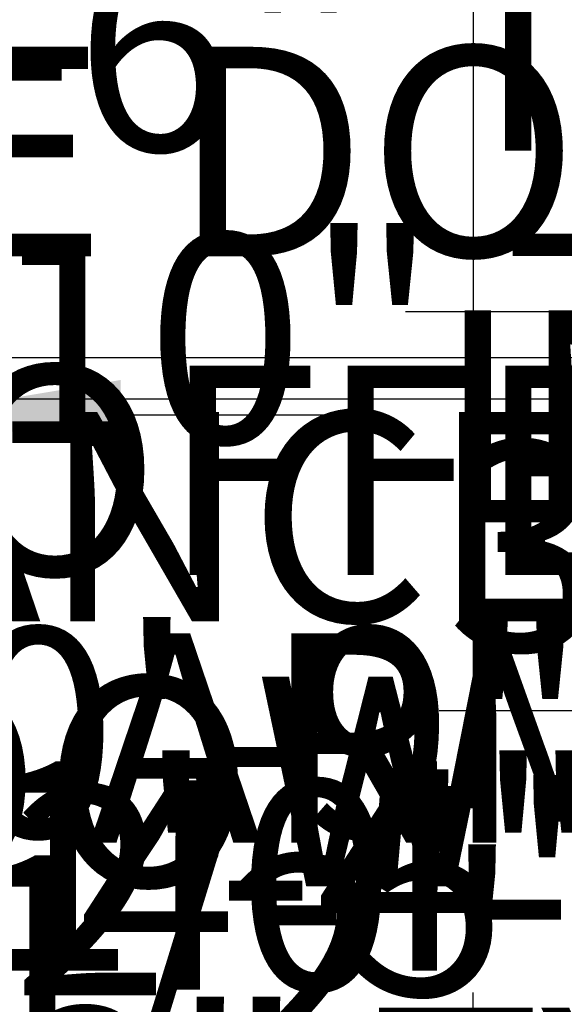
# Model space of a CAD drawing. Units: inches. Extents: x 7323 to 9737, y 2037 to 3322.
# Tile 9 of 19: x 8921 to 8999, y 2426 to 2568. Entities that reach past the tile are written whole.
import ezdxf

# ---------------------------------------------------------------- set-up
doc = ezdxf.new("R2010")
doc.units = ezdxf.units.IN
doc.header["$MEASUREMENT"] = 0
doc.layers.add('A-ANNO-DIMS', color=2, linetype='Continuous', lineweight=18)
doc.styles.get("Standard").update_dxf_attribs({"font": 'arial.ttf'})
doc.dimstyles.get("Standard").update_dxf_attribs({"dimtxt": 30.18, "dimasz": 30.18, "dimexe": 0.18, "dimexo": 0.0625, "dimgap": 0.09, "dimtad": 0, "dimtih": 1, "dimtoh": 1, "dimdec": 0, "dimzin": 0, "dimdsep": 46, "dimlunit": 3, "dimtxsty": 'Standard', "dimcen": 0.09, "dimadec": 0, "dimazin": 0, "dimtfac": 1, "dimtdec": 0, "dimtofl": 0, "dimtmove": 0, "dimatfit": 3, "dimfxl": 1, "dimtolj": 1, "dimtzin": 0, "dimarcsym": 0})

# ---------------------------------------------------------------- blocks, each defined once
blk = doc.blocks.new('*D11')
at = {"layer": 'A-ANNO-DIMS', "color": 0, "lineweight": -2, "transparency": 16777216}
for p, q in [((9007.88, 2687.3), (8985.8, 2687.3)), ((8985.98, 2657.12), (8985.98, 2458.79)), ((8985.98, 2229.48), (8985.98, 2427.8)), ((9007.88, 2199.3), (8985.8, 2199.3))]:
    blk.add_line(p, q, dxfattribs=at)
at = {"layer": 'A-ANNO-DIMS', "color": 0, "transparency": 16777216}
for points in [[(8980.95, 2657.12), (8991.01, 2657.12), (8985.98, 2687.3)], [(8980.95, 2229.48), (8991.01, 2229.48), (8985.98, 2199.3)]]:
    blk.add_solid(points, dxfattribs=at)
at = {"layer": 'Defpoints', "color": 0, "transparency": 16777216}
for p in [(9007.95, 2687.3), (8985.98, 2199.3), (9007.95, 2199.3)]:
    blk.add_point(p, dxfattribs=at)
at = {"layer": 'A-ANNO-DIMS', "color": 0, "transparency": 16777216, "insert": (8985.98, 2443.3), "char_height": 30.18, "attachment_point": 5}
blk.add_mtext('\\A1;40\'-8"', dxfattribs=at)
blk = doc.blocks.new('*D39')
at = {"layer": 'A-ANNO-DIMS', "color": 0, "lineweight": -2, "transparency": 16777216}
for p, q in [((8647.94, 2549.03), (8617.76, 2549.03)), ((8678.12, 2543.2), (8678.12, 2549.21)), ((8717.39, 2543.2), (8717.39, 2549.21)), ((8747.57, 2549.03), (8777.75, 2549.03))]:
    blk.add_line(p, q, dxfattribs=at)
at = {"layer": 'A-ANNO-DIMS', "color": 0, "transparency": 16777216}
for points in [[(8647.94, 2554.06), (8647.94, 2544), (8678.12, 2549.03)], [(8747.57, 2554.06), (8747.57, 2544), (8717.39, 2549.03)]]:
    blk.add_solid(points, dxfattribs=at)
at = {"layer": 'Defpoints', "color": 0, "transparency": 16777216}
for p in [(8717.39, 2549.03), (8678.12, 2543.14), (8717.39, 2543.14)]:
    blk.add_point(p, dxfattribs=at)
at = {"layer": 'A-ANNO-DIMS', "color": 0, "transparency": 16777216, "insert": (9057.19, 2549.03), "char_height": 30.18, "attachment_point": 5}
blk.add_mtext('\\A1;SINGLE DOOR 3\'-3 1/2" TYP.', dxfattribs=at)
blk = doc.blocks.new('*D41')
at = {"layer": 'A-ANNO-DIMS', "color": 0, "lineweight": -2, "transparency": 16777216}
for p, q in [((8661.59, 2428.04), (8661.59, 2458.22)), ((8661.59, 2458.22), (8691.77, 2458.22)), ((8657.46, 2397.86), (8661.77, 2397.86)), ((8657.46, 2369.86), (8661.77, 2369.86)), ((8661.59, 2339.68), (8661.59, 2309.5))]:
    blk.add_line(p, q, dxfattribs=at)
at = {"layer": 'A-ANNO-DIMS', "color": 0, "transparency": 16777216}
for points in [[(8656.56, 2428.04), (8666.62, 2428.04), (8661.59, 2397.86)], [(8656.56, 2339.68), (8666.62, 2339.68), (8661.59, 2369.86)]]:
    blk.add_solid(points, dxfattribs=at)
at = {"layer": 'Defpoints', "color": 0, "transparency": 16777216}
for p in [(8657.39, 2397.86), (8661.59, 2397.86), (8657.39, 2369.86)]:
    blk.add_point(p, dxfattribs=at)
at = {"layer": 'A-ANNO-DIMS', "color": 0, "transparency": 16777216, "insert": (8945.06, 2458.22), "char_height": 30.18, "attachment_point": 5}
blk.add_mtext('\\A1;VENT WINDOW 2\'-4" TYP.', dxfattribs=at)
blk = doc.blocks.new('*D43')
at = {"layer": 'A-ANNO-DIMS', "color": 0, "lineweight": -2, "transparency": 16777216}
for p, q in [((9108.94, 2438.75), (9108.94, 2468.93)), ((9104.01, 2408.57), (9109.12, 2408.57)), ((9104.01, 2375.3), (9109.12, 2375.3)), ((9108.94, 2345.12), (9108.94, 2314.94))]:
    blk.add_line(p, q, dxfattribs=at)
at = {"layer": 'A-ANNO-DIMS', "color": 0, "transparency": 16777216}
for points in [[(9103.91, 2438.75), (9113.97, 2438.75), (9108.94, 2408.57)], [(9103.91, 2345.12), (9113.97, 2345.12), (9108.94, 2375.3)]]:
    blk.add_solid(points, dxfattribs=at)
at = {"layer": 'Defpoints', "color": 0, "transparency": 16777216}
for p in [(9103.95, 2408.57), (9108.94, 2408.57), (9103.95, 2375.3)]:
    blk.add_point(p, dxfattribs=at)
at = {"layer": 'A-ANNO-DIMS', "color": 0, "transparency": 16777216, "insert": (9108.94, 2391.93), "char_height": 30.18, "attachment_point": 5}
blk.add_mtext('\\A1;BATH DOOR 2\'-9 1/2" TYP.', dxfattribs=at)
blk = doc.blocks.new('*D47')
at = {"layer": 'A-ANNO-DIMS', "color": 0, "lineweight": -2, "transparency": 16777216}
for p, q in [((8809.55, 2464.49), (8779.37, 2464.49)), ((8839.73, 2461.79), (8839.73, 2464.67)), ((8858.14, 2461.79), (8858.14, 2464.67)), ((8888.32, 2464.49), (8918.5, 2464.49))]:
    blk.add_line(p, q, dxfattribs=at)
at = {"layer": 'A-ANNO-DIMS', "color": 0, "transparency": 16777216}
for points in [[(8809.55, 2469.52), (8809.55, 2459.46), (8839.73, 2464.49)], [(8888.32, 2469.52), (8888.32, 2459.46), (8858.14, 2464.49)]]:
    blk.add_solid(points, dxfattribs=at)
at = {"layer": 'Defpoints', "color": 0, "transparency": 16777216}
for p in [(8858.14, 2464.49), (8839.73, 2461.73), (8858.14, 2461.73)]:
    blk.add_point(p, dxfattribs=at)
at = {"layer": 'A-ANNO-DIMS', "color": 0, "transparency": 16777216, "insert": (9164.9, 2464.49), "char_height": 30.18, "attachment_point": 5}
blk.add_mtext('\\A1;ARMCHAIR 1\'-6 1/2" TYP.', dxfattribs=at)
blk = doc.blocks.new('*D48')
at = {"layer": 'A-ANNO-DIMS', "color": 0, "lineweight": -2, "transparency": 16777216}
for p, q in [((8836.96, 2491.91), (8836.96, 2522.09)), ((8836.96, 2522.09), (8867.14, 2522.09)), ((8839.66, 2461.73), (8836.78, 2461.73)), ((8839.66, 2451.75), (8836.78, 2451.75)), ((8836.96, 2421.57), (8836.96, 2391.39))]:
    blk.add_line(p, q, dxfattribs=at)
at = {"layer": 'A-ANNO-DIMS', "color": 0, "transparency": 16777216}
for points in [[(8831.93, 2491.91), (8841.99, 2491.91), (8836.96, 2461.73)], [(8831.93, 2421.57), (8841.99, 2421.57), (8836.96, 2451.75)]]:
    blk.add_solid(points, dxfattribs=at)
at = {"layer": 'Defpoints', "color": 0, "transparency": 16777216}
for p in [(8836.96, 2461.73), (8839.73, 2461.73), (8839.73, 2451.75)]:
    blk.add_point(p, dxfattribs=at)
at = {"layer": 'A-ANNO-DIMS', "color": 0, "transparency": 16777216, "insert": (8970.94, 2522.09), "char_height": 30.18, "attachment_point": 5}
blk.add_mtext('\\A1;0\'-10" TYP.', dxfattribs=at)
blk = doc.blocks.new('*D53')
at = {"layer": 'A-ANNO-DIMS', "color": 0, "lineweight": -2, "transparency": 16777216}
for p, q in [((8826.85, 2511.06), (8796.67, 2511.06)), ((8857.03, 2503.93), (8857.03, 2511.24)), ((8905.03, 2503.93), (8905.03, 2511.24)), ((8935.21, 2511.06), (8965.39, 2511.06))]:
    blk.add_line(p, q, dxfattribs=at)
at = {"layer": 'A-ANNO-DIMS', "color": 0, "transparency": 16777216}
for points in [[(8826.85, 2516.09), (8826.85, 2506.03), (8857.03, 2511.06)], [(8935.21, 2516.09), (8935.21, 2506.03), (8905.03, 2511.06)]]:
    blk.add_solid(points, dxfattribs=at)
at = {"layer": 'Defpoints', "color": 0, "transparency": 16777216}
for p in [(8905.03, 2511.06), (8857.03, 2503.86), (8905.03, 2503.86)]:
    blk.add_point(p, dxfattribs=at)
at = {"layer": 'A-ANNO-DIMS', "color": 0, "transparency": 16777216, "insert": (9261.3, 2511.06), "char_height": 30.18, "attachment_point": 5}
blk.add_mtext('\\A1;INTERIOR WINDOW 4\'-0" TYP.', dxfattribs=at)
blk = doc.blocks.new('*D54')
at = {"layer": 'A-ANNO-DIMS', "color": 0, "lineweight": -2, "transparency": 16777216}
for p, q in [((8849.83, 2534.04), (8849.83, 2564.22)), ((8849.83, 2564.22), (8880.01, 2564.22)), ((8856.96, 2503.86), (8849.65, 2503.86)), ((8856.96, 2497.86), (8849.65, 2497.86)), ((8849.83, 2467.68), (8849.83, 2437.5))]:
    blk.add_line(p, q, dxfattribs=at)
at = {"layer": 'A-ANNO-DIMS', "color": 0, "transparency": 16777216}
for points in [[(8844.8, 2534.04), (8854.86, 2534.04), (8849.83, 2503.86)], [(8844.8, 2467.68), (8854.86, 2467.68), (8849.83, 2497.86)]]:
    blk.add_solid(points, dxfattribs=at)
at = {"layer": 'Defpoints', "color": 0, "transparency": 16777216}
for p in [(8849.83, 2503.86), (8857.03, 2503.86), (8857.03, 2497.86)]:
    blk.add_point(p, dxfattribs=at)
at = {"layer": 'A-ANNO-DIMS', "color": 0, "transparency": 16777216, "insert": (8972.08, 2564.22), "char_height": 30.18, "attachment_point": 5}
blk.add_mtext('\\A1;0\'-6" TYP.', dxfattribs=at)
blk = doc.blocks.new('*D60')
at = {"layer": 'A-ANNO-DIMS', "color": 0, "lineweight": -2, "transparency": 16777216}
for p, q in [((9109.84, 2540.48), (9109.84, 2570.66)), ((9104.01, 2510.3), (9110.02, 2510.3)), ((9104.01, 2474.02), (9110.02, 2474.02)), ((9109.84, 2443.84), (9109.84, 2413.66))]:
    blk.add_line(p, q, dxfattribs=at)
at = {"layer": 'A-ANNO-DIMS', "color": 0, "transparency": 16777216}
for points in [[(9104.81, 2540.48), (9114.87, 2540.48), (9109.84, 2510.3)], [(9104.81, 2443.84), (9114.87, 2443.84), (9109.84, 2474.02)]]:
    blk.add_solid(points, dxfattribs=at)
at = {"layer": 'Defpoints', "color": 0, "transparency": 16777216}
for p in [(9103.95, 2510.3), (9109.84, 2510.3), (9103.95, 2474.02)]:
    blk.add_point(p, dxfattribs=at)
at = {"layer": 'A-ANNO-DIMS', "color": 0, "transparency": 16777216, "insert": (9109.84, 2492.16), "char_height": 30.18, "attachment_point": 5}
blk.add_mtext('\\A1;3\'-0 1/2" TYP.', dxfattribs=at)
blk = doc.blocks.new('*D63')
at = {"layer": 'A-ANNO-DIMS', "color": 0, "lineweight": -2, "transparency": 16777216}
for p, q in [((8744.72, 2466.22), (8744.72, 2496.4)), ((8744.72, 2496.4), (8774.9, 2496.4)), ((8741.46, 2436.04), (8744.9, 2436.04)), ((8741.46, 2413.86), (8744.9, 2413.86)), ((8744.72, 2383.68), (8744.72, 2353.5))]:
    blk.add_line(p, q, dxfattribs=at)
at = {"layer": 'A-ANNO-DIMS', "color": 0, "transparency": 16777216}
for points in [[(8739.69, 2466.22), (8749.75, 2466.22), (8744.72, 2436.04)], [(8739.69, 2383.68), (8749.75, 2383.68), (8744.72, 2413.86)]]:
    blk.add_solid(points, dxfattribs=at)
at = {"layer": 'Defpoints', "color": 0, "transparency": 16777216}
for p in [(8741.39, 2436.04), (8744.72, 2436.04), (8741.39, 2413.86)]:
    blk.add_point(p, dxfattribs=at)
at = {"layer": 'A-ANNO-DIMS', "color": 0, "transparency": 16777216, "insert": (9003.76, 2496.4), "char_height": 30.18, "attachment_point": 5}
blk.add_mtext('\\A1;APPLIANCE 1\'-10" TYP.', dxfattribs=at)
blk = doc.blocks.new('*D64')
at = {"layer": 'A-ANNO-DIMS', "color": 0, "lineweight": -2, "transparency": 16777216}
for p, q in [((8719.69, 2413.8), (8719.69, 2410.36)), ((8741.39, 2413.8), (8741.39, 2410.36)), ((8689.51, 2410.54), (8659.33, 2410.54)), ((8771.57, 2410.54), (8801.75, 2410.54))]:
    blk.add_line(p, q, dxfattribs=at)
at = {"layer": 'A-ANNO-DIMS', "color": 0, "transparency": 16777216}
for points in [[(8689.51, 2415.57), (8689.51, 2405.51), (8719.69, 2410.54)], [(8771.57, 2415.57), (8771.57, 2405.51), (8741.39, 2410.54)]]:
    blk.add_solid(points, dxfattribs=at)
at = {"layer": 'Defpoints', "color": 0, "transparency": 16777216}
for p in [(8719.69, 2413.86), (8741.39, 2413.86), (8741.39, 2410.54)]:
    blk.add_point(p, dxfattribs=at)
at = {"layer": 'A-ANNO-DIMS', "color": 0, "transparency": 16777216, "insert": (8927.57, 2410.54), "char_height": 30.18, "attachment_point": 5}
blk.add_mtext('\\A1;1\'-9 1/2" TYP.', dxfattribs=at)
blk = doc.blocks.new('*D66')
at = {"layer": 'A-ANNO-DIMS', "color": 0, "lineweight": -2, "transparency": 16777216}
for p, q in [((9036.62, 2513.36), (9036.62, 2526.08)), ((9075.95, 2513.36), (9075.95, 2526.08)), ((9006.44, 2525.9), (8976.26, 2525.9)), ((9106.13, 2525.9), (9136.31, 2525.9))]:
    blk.add_line(p, q, dxfattribs=at)
at = {"layer": 'A-ANNO-DIMS', "color": 0, "transparency": 16777216}
for points in [[(9006.44, 2530.93), (9006.44, 2520.87), (9036.62, 2525.9)], [(9106.13, 2530.93), (9106.13, 2520.87), (9075.95, 2525.9)]]:
    blk.add_solid(points, dxfattribs=at)
at = {"layer": 'Defpoints', "color": 0, "transparency": 16777216}
for p in [(9075.95, 2525.9), (9036.62, 2513.3), (9075.95, 2513.3)]:
    blk.add_point(p, dxfattribs=at)
at = {"layer": 'A-ANNO-DIMS', "color": 0, "transparency": 16777216, "insert": (9263.53, 2525.9), "char_height": 30.18, "attachment_point": 5}
blk.add_mtext('\\A1;3\'-3 1/2" TYP.', dxfattribs=at)
blk = doc.blocks.new('*D69')
at = {"layer": 'A-ANNO-DIMS', "color": 0, "lineweight": -2, "transparency": 16777216}
for p, q in [((8836.58, 2472.89), (8836.58, 2503.07)), ((8836.58, 2503.07), (8866.76, 2503.07)), ((8839.88, 2442.71), (8836.4, 2442.71)), ((8839.88, 2420.33), (8836.4, 2420.33)), ((8836.58, 2390.15), (8836.58, 2359.97))]:
    blk.add_line(p, q, dxfattribs=at)
at = {"layer": 'A-ANNO-DIMS', "color": 0, "transparency": 16777216}
for points in [[(8831.55, 2472.89), (8841.61, 2472.89), (8836.58, 2442.71)], [(8831.55, 2390.15), (8841.61, 2390.15), (8836.58, 2420.33)]]:
    blk.add_solid(points, dxfattribs=at)
at = {"layer": 'Defpoints', "color": 0, "transparency": 16777216}
for p in [(8836.58, 2442.71), (8839.94, 2442.71), (8839.94, 2420.33)]:
    blk.add_point(p, dxfattribs=at)
at = {"layer": 'A-ANNO-DIMS', "color": 0, "transparency": 16777216, "insert": (9169.54, 2503.07), "char_height": 30.18, "attachment_point": 5}
blk.add_mtext('\\A1;COFFEE TABLE 1\'-10 1/2" TYP.', dxfattribs=at)
blk = doc.blocks.new('*D70')
at = {"layer": 'A-ANNO-DIMS', "color": 0, "lineweight": -2, "transparency": 16777216}
for p, q in [((8809.76, 2446.06), (8779.58, 2446.06)), ((8839.94, 2442.77), (8839.94, 2446.24)), ((8855.74, 2442.77), (8855.74, 2446.24)), ((8885.92, 2446.06), (8916.1, 2446.06))]:
    blk.add_line(p, q, dxfattribs=at)
at = {"layer": 'A-ANNO-DIMS', "color": 0, "transparency": 16777216}
for points in [[(8809.76, 2451.09), (8809.76, 2441.03), (8839.94, 2446.06)], [(8885.92, 2451.09), (8885.92, 2441.03), (8855.74, 2446.06)]]:
    blk.add_solid(points, dxfattribs=at)
at = {"layer": 'Defpoints', "color": 0, "transparency": 16777216}
for p in [(8855.74, 2446.06), (8839.94, 2442.71), (8855.74, 2442.71)]:
    blk.add_point(p, dxfattribs=at)
at = {"layer": 'A-ANNO-DIMS', "color": 0, "transparency": 16777216, "insert": (9006.75, 2446.06), "char_height": 30.18, "attachment_point": 5}
blk.add_mtext('\\A1;1\'-4" TYP.', dxfattribs=at)
blk = doc.blocks.new('*D71')
at = {"layer": 'A-ANNO-DIMS', "color": 0, "lineweight": -2, "transparency": 16777216}
for p, q in [((8891.18, 2486.02), (8891.18, 2516.2)), ((8884.24, 2455.84), (8891.36, 2455.84)), ((8884.24, 2409.18), (8891.36, 2409.18)), ((8891.18, 2379), (8891.18, 2348.82))]:
    blk.add_line(p, q, dxfattribs=at)
at = {"layer": 'A-ANNO-DIMS', "color": 0, "transparency": 16777216}
for points in [[(8886.15, 2486.02), (8896.21, 2486.02), (8891.18, 2455.84)], [(8886.15, 2379), (8896.21, 2379), (8891.18, 2409.18)]]:
    blk.add_solid(points, dxfattribs=at)
at = {"layer": 'Defpoints', "color": 0, "transparency": 16777216}
for p in [(8884.18, 2455.84), (8891.18, 2455.84), (8884.18, 2409.18)]:
    blk.add_point(p, dxfattribs=at)
at = {"layer": 'A-ANNO-DIMS', "color": 0, "transparency": 16777216, "insert": (8891.18, 2432.51), "char_height": 30.18, "attachment_point": 5}
blk.add_mtext('\\A1;SOFA 3\'-10 1/2" TYP.', dxfattribs=at)
blk = doc.blocks.new('*D72')
at = {"layer": 'A-ANNO-DIMS', "color": 0, "lineweight": -2, "transparency": 16777216}
for p, q in [((8864.06, 2409.12), (8864.06, 2402)), ((8884.18, 2409.12), (8884.18, 2402)), ((8833.88, 2402.18), (8803.7, 2402.18)), ((8914.36, 2402.18), (8944.54, 2402.18))]:
    blk.add_line(p, q, dxfattribs=at)
at = {"layer": 'A-ANNO-DIMS', "color": 0, "transparency": 16777216}
for points in [[(8833.88, 2407.21), (8833.88, 2397.15), (8864.06, 2402.18)], [(8914.36, 2407.21), (8914.36, 2397.15), (8884.18, 2402.18)]]:
    blk.add_solid(points, dxfattribs=at)
at = {"layer": 'Defpoints', "color": 0, "transparency": 16777216}
for p in [(8864.06, 2409.18), (8884.18, 2409.18), (8884.18, 2402.18)]:
    blk.add_point(p, dxfattribs=at)
at = {"layer": 'A-ANNO-DIMS', "color": 0, "transparency": 16777216, "insert": (9035.19, 2402.18), "char_height": 30.18, "attachment_point": 5}
blk.add_mtext('\\A1;1\'-8" TYP.', dxfattribs=at)
blk = doc.blocks.new('*D79')
at = {"layer": 'A-ANNO-DIMS', "color": 0, "lineweight": -2, "transparency": 16777216}
for p, q in [((8871.1, 2395.97), (8871.1, 2394.46)), ((8880.36, 2395.97), (8880.36, 2394.46)), ((8840.92, 2394.64), (8810.74, 2394.64)), ((8910.54, 2394.64), (8940.72, 2394.64))]:
    blk.add_line(p, q, dxfattribs=at)
at = {"layer": 'A-ANNO-DIMS', "color": 0, "transparency": 16777216}
for points in [[(8840.92, 2399.67), (8840.92, 2389.61), (8871.1, 2394.64)], [(8910.54, 2399.67), (8910.54, 2389.61), (8880.36, 2394.64)]]:
    blk.add_solid(points, dxfattribs=at)
at = {"layer": 'Defpoints', "color": 0, "transparency": 16777216}
for p in [(8871.1, 2396.03), (8880.36, 2396.03), (8880.36, 2394.64)]:
    blk.add_point(p, dxfattribs=at)
at = {"layer": 'A-ANNO-DIMS', "color": 0, "transparency": 16777216, "insert": (9195.57, 2394.64), "char_height": 30.18, "attachment_point": 5}
blk.add_mtext('\\A1;SIDE TABLE 0\'-9 1/2" TYP.', dxfattribs=at)
blk = doc.blocks.new('*D80')
at = {"layer": 'A-ANNO-DIMS', "color": 0, "lineweight": -2, "transparency": 16777216}
for p, q in [((8881.74, 2435.12), (8881.74, 2465.3)), ((8881.74, 2465.3), (8911.92, 2465.3)), ((8880.42, 2404.94), (8881.92, 2404.94)), ((8880.42, 2396.03), (8881.92, 2396.03)), ((8881.74, 2365.85), (8881.74, 2335.67))]:
    blk.add_line(p, q, dxfattribs=at)
at = {"layer": 'A-ANNO-DIMS', "color": 0, "transparency": 16777216}
for points in [[(8876.71, 2435.12), (8886.77, 2435.12), (8881.74, 2404.94)], [(8876.71, 2365.85), (8886.77, 2365.85), (8881.74, 2396.03)]]:
    blk.add_solid(points, dxfattribs=at)
at = {"layer": 'Defpoints', "color": 0, "transparency": 16777216}
for p in [(8880.36, 2404.94), (8881.74, 2404.94), (8880.36, 2396.03)]:
    blk.add_point(p, dxfattribs=at)
at = {"layer": 'A-ANNO-DIMS', "color": 0, "transparency": 16777216, "insert": (9003.99, 2465.3), "char_height": 30.18, "attachment_point": 5}
blk.add_mtext('\\A1;0\'-9" TYP.', dxfattribs=at)
blk = doc.blocks.new('*D100')
at = {"layer": 'A-ANNO-DIMS', "color": 0, "lineweight": -2, "transparency": 16777216}
for p, q in [((9007.88, 2687.3), (8587.16, 2687.3)), ((8587.34, 2657.12), (8587.34, 2615.8)), ((8587.34, 2543.49), (8587.34, 2584.8)), ((9008.12, 2513.31), (8587.16, 2513.31))]:
    blk.add_line(p, q, dxfattribs=at)
at = {"layer": 'A-ANNO-DIMS', "color": 0, "transparency": 16777216}
for points in [[(8582.31, 2657.12), (8592.37, 2657.12), (8587.34, 2687.3)], [(8582.31, 2543.49), (8592.37, 2543.49), (8587.34, 2513.31)]]:
    blk.add_solid(points, dxfattribs=at)
at = {"layer": 'Defpoints', "color": 0, "transparency": 16777216}
for p in [(9007.95, 2687.3), (8587.34, 2513.31), (9008.18, 2513.31)]:
    blk.add_point(p, dxfattribs=at)
at = {"layer": 'A-ANNO-DIMS', "color": 0, "transparency": 16777216, "insert": (8587.34, 2600.3), "char_height": 30.18, "attachment_point": 5}
blk.add_mtext('\\A1;14\'-6"', dxfattribs=at)
blk = doc.blocks.new('*D106')
at = {"layer": 'A-ANNO-DIMS', "color": 0, "lineweight": -2, "transparency": 16777216}
for p, q in [((9008.12, 2519.31), (8587.16, 2519.31)), ((8587.34, 2489.13), (8587.34, 2439.14)), ((8587.34, 2357.76), (8587.34, 2407.75)), ((9008.23, 2327.58), (8587.16, 2327.58))]:
    blk.add_line(p, q, dxfattribs=at)
at = {"layer": 'A-ANNO-DIMS', "color": 0, "transparency": 16777216}
for points in [[(8582.31, 2489.13), (8592.37, 2489.13), (8587.34, 2519.31)], [(8582.31, 2357.76), (8592.37, 2357.76), (8587.34, 2327.58)]]:
    blk.add_solid(points, dxfattribs=at)
at = {"layer": 'Defpoints', "color": 0, "transparency": 16777216}
for p in [(8587.34, 2519.31), (9008.18, 2519.31), (9008.29, 2327.58)]:
    blk.add_point(p, dxfattribs=at)
at = {"layer": 'A-ANNO-DIMS', "color": 0, "transparency": 16777216, "insert": (8587.34, 2423.44), "char_height": 30.18, "attachment_point": 5}
blk.add_mtext('\\A1;15\'-11 1/2"', dxfattribs=at)
blk = doc.blocks.new('*D110')
at = {"layer": 'A-ANNO-DIMS', "color": 0, "lineweight": -2, "transparency": 16777216}
for p, q in [((8587.34, 2449.91), (8587.34, 2480.09)), ((9018.85, 2419.73), (8587.16, 2419.73)), ((9018.85, 2375.3), (8587.16, 2375.3)), ((8587.34, 2345.12), (8587.34, 2314.94))]:
    blk.add_line(p, q, dxfattribs=at)
at = {"layer": 'A-ANNO-DIMS', "color": 0, "transparency": 16777216}
for points in [[(8582.31, 2449.91), (8592.37, 2449.91), (8587.34, 2419.73)], [(8582.31, 2345.12), (8592.37, 2345.12), (8587.34, 2375.3)]]:
    blk.add_solid(points, dxfattribs=at)
at = {"layer": 'Defpoints', "color": 0, "transparency": 16777216}
for p in [(8587.34, 2419.73), (9018.91, 2419.73), (9018.91, 2375.3)]:
    blk.add_point(p, dxfattribs=at)
at = {"layer": 'A-ANNO-DIMS', "color": 0, "transparency": 16777216, "insert": (8587.34, 2397.51), "char_height": 30.18, "attachment_point": 5}
blk.add_mtext('\\A1;3\'-8 1/2"', dxfattribs=at)
blk = doc.blocks.new('*D111')
at = {"layer": 'A-ANNO-DIMS', "color": 0, "lineweight": -2, "transparency": 16777216}
for p, q in [((9011.299226, 2468.388949), (8981.119226, 2468.388949)), ((9041.479226, 2433.251449), (9041.479226, 2468.568949)), ((9066.478924, 2433.251449), (9066.478924, 2468.568949)), ((9096.658924, 2468.388949), (9126.838924, 2468.388949))]:
    blk.add_line(p, q, dxfattribs=at)
at = {"layer": 'A-ANNO-DIMS', "color": 0, "transparency": 16777216}
for points in [[(9011.299226, 2473.418949), (9011.299226, 2463.358949), (9041.479226, 2468.388949)], [(9096.658924, 2473.418949), (9096.658924, 2463.358949), (9066.478924, 2468.388949)]]:
    blk.add_solid(points, dxfattribs=at)
at = {"layer": 'Defpoints', "color": 0, "transparency": 16777216}
for p in [(9066.478924, 2468.388949), (9041.479226, 2433.188949), (9066.478924, 2433.188949)]:
    blk.add_point(p, dxfattribs=at)
at = {"layer": 'A-ANNO-DIMS', "color": 0, "transparency": 16777216, "insert": (9167.299306, 2468.388949), "char_height": 30.18, "attachment_point": 5}
blk.add_mtext('\\A1;2\'-1"', dxfattribs=at)
blk = doc.blocks.new('*D114')
at = {"layer": 'A-ANNO-DIMS', "color": 0, "lineweight": -2, "transparency": 16777216}
for p, q in [((8915.46, 2671.86), (9307.45, 2671.86)), ((9307.27, 2641.68), (9307.27, 2641.04)), ((8915.46, 2610.86), (9307.45, 2610.86)), ((9307.27, 2610.86), (9307.27, 2580.68)), ((9307.27, 2580.68), (9277.09, 2580.68))]:
    blk.add_line(p, q, dxfattribs=at)
at = {"layer": 'A-ANNO-DIMS', "color": 0, "transparency": 16777216}
for points in [[(9302.24, 2641.68), (9312.3, 2641.68), (9307.27, 2671.86)], [(9302.24, 2641.04), (9312.3, 2641.04), (9307.27, 2610.86)]]:
    blk.add_solid(points, dxfattribs=at)
at = {"layer": 'Defpoints', "color": 0, "transparency": 16777216}
for p in [(8915.39, 2671.86), (8915.39, 2610.86), (9307.27, 2610.86)]:
    blk.add_point(p, dxfattribs=at)
at = {"layer": 'A-ANNO-DIMS', "color": 0, "transparency": 16777216, "insert": (9236.89, 2580.68), "char_height": 30.18, "attachment_point": 5}
blk.add_mtext('\\A1;5\'-1"', dxfattribs=at)
blk = doc.blocks.new('*D126')
at = {"layer": 'A-ANNO-DIMS', "color": 0, "lineweight": -2, "transparency": 16777216}
for p, q in [((9109.28, 2586.63), (9139.46, 2586.63)), ((9139.46, 2586.63), (9160.18, 2564.69)), ((9204.86, 2517.3), (9205.04, 2517.3)), ((9204.95, 2517.21), (9204.95, 2517.39))]:
    blk.add_line(p, q, dxfattribs=at)
at = {"layer": 'A-ANNO-DIMS', "color": 0, "transparency": 16777216}
blk.add_solid([(9163.84, 2568.15), (9156.52, 2561.24), (9180.9, 2542.75)], dxfattribs=at)
at = {"layer": 'Defpoints', "color": 0, "transparency": 16777216}
for p in [(9180.9, 2542.75), (9204.95, 2517.3)]:
    blk.add_point(p, dxfattribs=at)
at = {"layer": 'A-ANNO-DIMS', "color": 0, "transparency": 16777216, "insert": (9009.88, 2586.63), "char_height": 30.18, "attachment_point": 5}
blk.add_mtext('\\A1;4X R2\'-11"', dxfattribs=at)
blk = doc.blocks.new('*D127')
at = {"layer": 'A-ANNO-DIMS', "color": 0, "lineweight": -2, "transparency": 16777216}
for p, q in [((9006.57, 2442.49), (9036.75, 2442.49)), ((9036.75, 2442.49), (9058.09, 2421.15)), ((9099.86, 2379.3), (9100.04, 2379.3)), ((9099.95, 2379.21), (9099.95, 2379.39))]:
    blk.add_line(p, q, dxfattribs=at)
at = {"layer": 'A-ANNO-DIMS', "color": 0, "transparency": 16777216}
blk.add_solid([(9061.64, 2424.71), (9054.53, 2417.6), (9079.43, 2399.81)], dxfattribs=at)
at = {"layer": 'Defpoints', "color": 0, "transparency": 16777216}
for p in [(9079.43, 2399.81), (9099.95, 2379.3)]:
    blk.add_point(p, dxfattribs=at)
at = {"layer": 'A-ANNO-DIMS', "color": 0, "transparency": 16777216, "insert": (8951.92, 2442.49), "char_height": 30.18, "attachment_point": 5}
blk.add_mtext('\\A1;R2\'-5"', dxfattribs=at)

msp = doc.modelspace()

# ---------------------------------------------------------------- dimensions: what is measured, and where the dimension line sits
at = {"layer": 'A-ANNO-DIMS'}
for base, p1, p2, override, picture, middle in [((8587.34, 2513.31), (9007.95, 2687.3), (9008.18, 2513.31), {"dimdec": 1, "dimlfac": 1, "dimrnd": 0, "dimzin": 1, "dimdsep": 46, "dimlunit": 4, "dimfrac": 2}, '*D100', (8587.34, 2600.3)), ((8985.98, 2199.3), (9007.95, 2687.3), (9007.95, 2199.3), {"dimclrd": 0, "dimclre": 0, "dimclrt": 0}, '*D11', (8985.98, 2443.3)), ((9307.27, 2610.86), (8915.39, 2671.86), (8915.39, 2610.86), {"dimdec": 1, "dimlfac": 1, "dimrnd": 0, "dimzin": 1, "dimdsep": 46, "dimlunit": 4, "dimfrac": 2}, '*D114', (9236.89, 2580.68)), ((8587.34, 2519.31), (9008.29, 2327.58), (9008.18, 2519.31), {"dimdec": 1, "dimlfac": 1, "dimrnd": 0, "dimzin": 1, "dimdsep": 46, "dimlunit": 4, "dimfrac": 2}, '*D106', (8587.34, 2423.44)), ((8587.34, 2419.73), (9018.91, 2375.3), (9018.91, 2419.73), {"dimdec": 1, "dimlfac": 1, "dimrnd": 0, "dimzin": 1, "dimdsep": 46, "dimlunit": 4, "dimfrac": 2}, '*D110', (8587.34, 2397.51))]:
    dim = msp.add_linear_dim(base=base, p1=p1, p2=p2, angle=90, dimstyle='Standard', override=override, dxfattribs=at)
    dim.commit()
    dim.dimension.update_dxf_attribs({"geometry": picture, "text_midpoint": middle})
for base, p1, p2, text, picture, middle in [((8717.39, 2549.03), (8678.12, 2543.14), (8717.39, 2543.14), 'SINGLE DOOR <> TYP.', '*D39', (9057.19, 2549.03)), ((8905.03, 2511.06), (8857.03, 2503.86), (8905.03, 2503.86), 'INTERIOR WINDOW <> TYP.', '*D53', (9261.3, 2511.06)), ((9075.95, 2525.9), (9036.62, 2513.3), (9075.95, 2513.3), '<> TYP.', '*D66', (9263.53, 2525.9)), ((8858.14, 2464.49), (8839.73, 2461.73), (8858.14, 2461.73), 'ARMCHAIR <> TYP.', '*D47', (9164.9, 2464.49)), ((8880.36, 2394.64), (8871.1, 2396.03), (8880.36, 2396.03), 'SIDE TABLE <> TYP.', '*D79', (9195.57, 2394.64)), ((8855.74, 2446.06), (8839.94, 2442.71), (8855.74, 2442.71), '<> TYP.', '*D70', (9006.75, 2446.06)), ((8741.39, 2410.54), (8719.69, 2413.86), (8741.39, 2413.86), '<> TYP.', '*D64', (8927.57, 2410.54)), ((8884.18, 2402.18), (8864.06, 2409.18), (8884.18, 2409.18), '<> TYP.', '*D72', (9035.19, 2402.18))]:
    dim = msp.add_linear_dim(base=base, p1=p1, p2=p2, text=text, dimstyle='Standard', override={"dimdec": 1, "dimlfac": 1, "dimrnd": 0, "dimzin": 1, "dimdsep": 46, "dimlunit": 4, "dimfrac": 2}, dxfattribs=at)
    dim.commit()
    dim.dimension.update_dxf_attribs({"geometry": picture, "text_midpoint": middle})
dim = msp.add_radius_dim(center=(9204.95, 2517.3), mpoint=(9180.9, 2542.75), text='4X <>', dimstyle='Standard', override={"dimdec": 1, "dimlfac": 1, "dimrnd": 0, "dimzin": 1, "dimdsep": 46, "dimlunit": 4, "dimfrac": 2}, dxfattribs=at)
dim.commit()
dim.dimension.update_dxf_attribs({"geometry": '*D126', "text_midpoint": (9009.88, 2586.63)})
for base, p1, p2, text, picture, middle in [((8836.58, 2442.71), (8839.94, 2420.33), (8839.94, 2442.71), 'COFFEE TABLE <> TYP.', '*D69', (9169.54, 2503.07)), ((8849.83, 2503.86), (8857.03, 2497.86), (8857.03, 2503.86), '<> TYP.', '*D54', (8972.08, 2564.22)), ((9109.84, 2510.3), (9103.95, 2474.02), (9103.95, 2510.3), '<> TYP.', '*D60', (9109.84, 2492.16)), ((8744.72, 2436.04), (8741.39, 2413.86), (8741.39, 2436.04), 'APPLIANCE <> TYP.', '*D63', (9003.76, 2496.4)), ((8836.96, 2461.73), (8839.73, 2451.75), (8839.73, 2461.73), '<> TYP.', '*D48', (8970.94, 2522.09)), ((8661.59, 2397.86), (8657.39, 2369.86), (8657.39, 2397.86), 'VENT WINDOW <> TYP.', '*D41', (8945.06, 2458.22)), ((8891.18, 2455.84), (8884.18, 2409.18), (8884.18, 2455.84), 'SOFA <> TYP.', '*D71', (8891.18, 2432.51)), ((9108.94, 2408.57), (9103.95, 2375.3), (9103.95, 2408.57), 'BATH DOOR <> TYP.', '*D43', (9108.94, 2391.93)), ((8881.74, 2404.94), (8880.36, 2396.03), (8880.36, 2404.94), '<> TYP.', '*D80', (9003.99, 2465.3))]:
    dim = msp.add_linear_dim(base=base, p1=p1, p2=p2, angle=90, text=text, dimstyle='Standard', override={"dimdec": 1, "dimlfac": 1, "dimrnd": 0, "dimzin": 1, "dimdsep": 46, "dimlunit": 4, "dimfrac": 2}, dxfattribs=at)
    dim.commit()
    dim.dimension.update_dxf_attribs({"geometry": picture, "text_midpoint": middle})
dim = msp.add_linear_dim(base=(9066.48, 2468.39), p1=(9041.48, 2433.19), p2=(9066.48, 2433.19), dimstyle='Standard', override={"dimdec": 1, "dimlfac": 1, "dimrnd": 0, "dimzin": 1, "dimdsep": 46, "dimlunit": 4, "dimfrac": 2}, dxfattribs=at)
dim.commit()
dim.dimension.update_dxf_attribs({"geometry": '*D111', "text_midpoint": (9167.3, 2468.39)})
dim = msp.add_radius_dim(center=(9099.95, 2379.3), mpoint=(9079.43, 2399.81), dimstyle='Standard', override={"dimdec": 1, "dimlfac": 1, "dimrnd": 0, "dimzin": 1, "dimdsep": 46, "dimlunit": 4, "dimfrac": 2}, dxfattribs=at)
dim.commit()
dim.dimension.update_dxf_attribs({"geometry": '*D127', "text_midpoint": (8951.92, 2442.49)})

doc.saveas('drawing.dxf')
